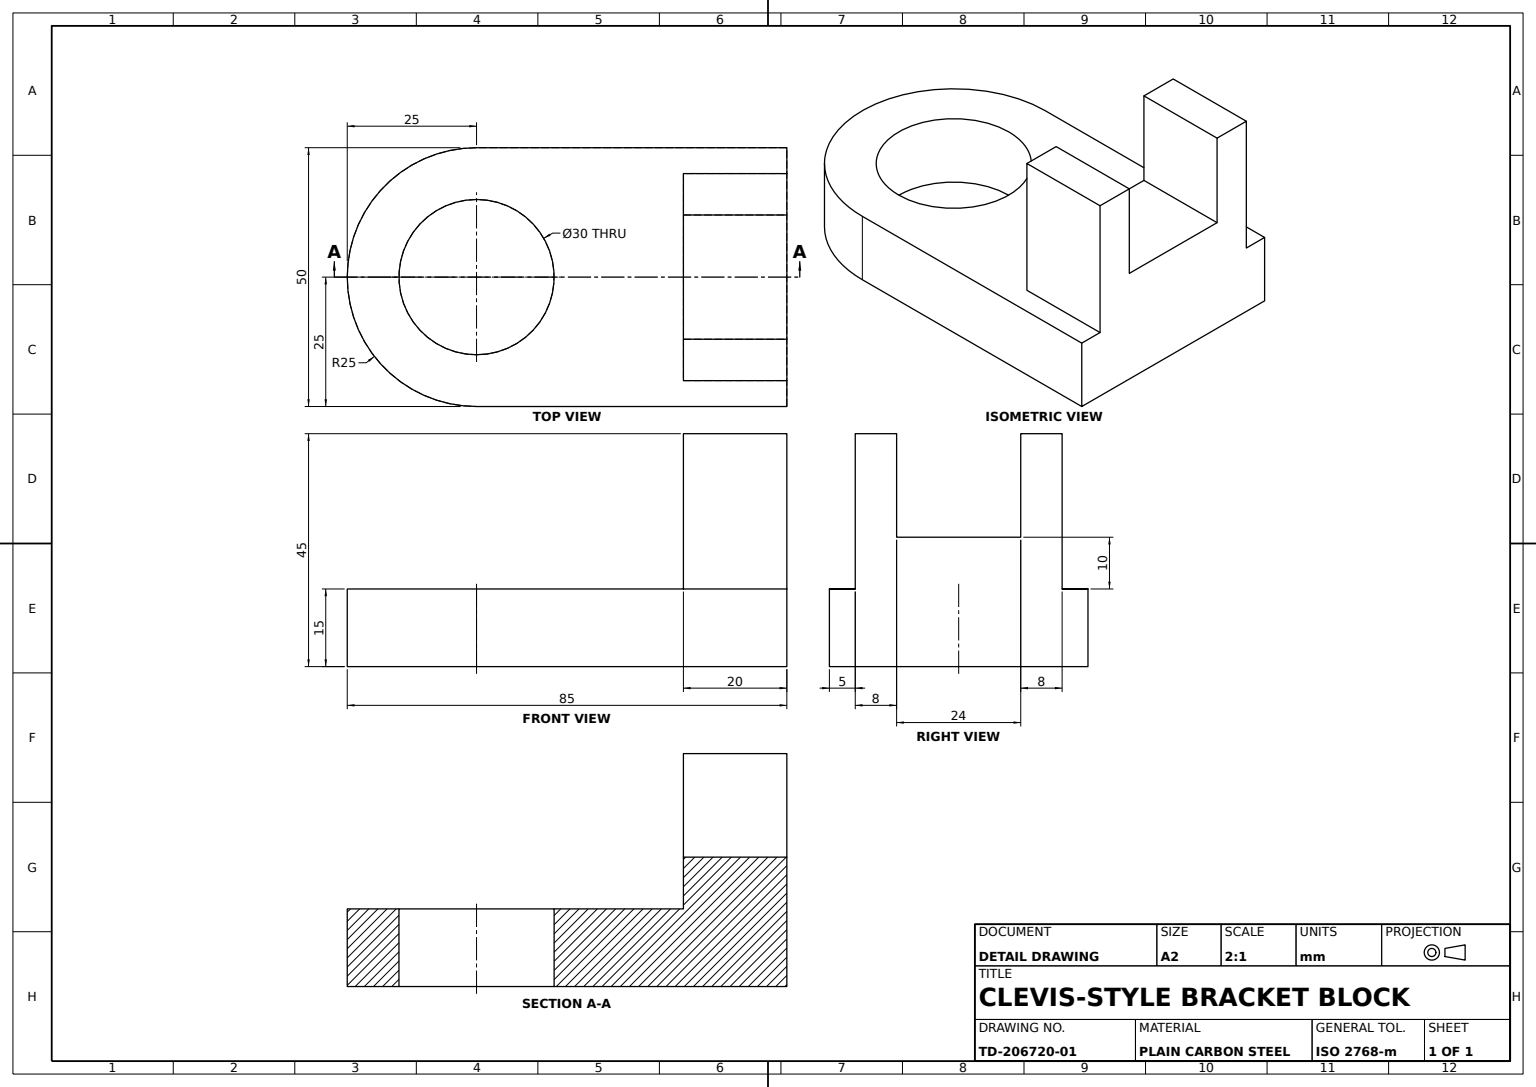
SolidWorks part; units mm, degrees
material "Plain Carbon Steel"
ref_plane "Front Plane" through (0, 0, 0) normal (0, 0, 1) x (1, 0, 0)
ref_plane "Top Plane" through (0, 0, 0) normal (0, 1, 0) x (1, 0, 0)
ref_plane "Right Plane" through (0, 0, 0) normal (1, 0, 0) x (0, 0, -1)
sketch "Base Block Sketch" plane through (0, 0, 0) normal (0, 0, 1) x (1, 0, 0)
  line L1 (-30, 7.5) -> (30, 7.5)
  line L2 (-30, 7.5) -> (-30, -7.5)
  line L3 (-30, -7.5) -> (30, -7.5)
  line L4 (30, 7.5) -> (30, -7.5)
  point P0 (0, 0)
  dimension "D1" = 60
  dimension "D2" = 15
  dimension "D3" = 7.5
  dimension "D4" = 30
extrude "Base Block" add sketch "Base Block Sketch" along normal mid plane 50
sketch "Fork Upright Sketch" plane through (30, 0, 0) normal (1, 0, 0) x (0, 0, -1)
  line L1 (-25, 7.5) -> (25, 7.5) construction
  line L2 (-20, 7.5) -> (-20, 37.5)
  line L3 (-20, 37.5) -> (-12, 37.5)
  line L4 (-12, 37.5) -> (-12, 17.5)
  line L5 (-12, 17.5) -> (12, 17.5)
  line L6 (12, 17.5) -> (12, 37.5)
  line L7 (12, 37.5) -> (20, 37.5)
  line L8 (20, 37.5) -> (20, 7.5)
  line L9 (20, 7.5) -> (-20, 7.5)
  dimension "D1" = 24
  dimension "D2" = 8
  dimension "D3" = 30
  dimension "D4" = 17.5
  dimension "D5" = 8
  dimension "D6" = 21.36
  dimension "D7" = 37.5
extrude "Fork Upright" add sketch "Fork Upright Sketch" against normal blind 20
sketch "End Lug Sketch" plane through (0, 7.5, 0) normal (0, 1, 0) x (1, 0, 0)
  line L1 (-30, -25) -> (-30, 25) construction
  line L2 (-30, 25) -> (-30, -25)
  arc A1 (-30, 15) -> (-30, -15) centre (-30, 0) ccw
  arc A2 (-30, 25) -> (-30, -25) centre (-30, 0) ccw
  line M6 (-30, 25) -> (-30, -25)
  dimension "D1" = 15
extrude "Rounded End Lug" add sketch "End Lug Sketch" against normal blind 15 contours A2 A1 M6
sketch "Bore Sketch" plane through (0, 7.5, 0) normal (0, 1, 0) x (1, 0, 0)
  line L0 (-30, -15) -> (-30, 15) construction
  circle A0 centre (-30, 0) radius 15
  dimension "D1" = 30
extrude "Bore Ø30" cut sketch "Bore Sketch" against normal blind 15
